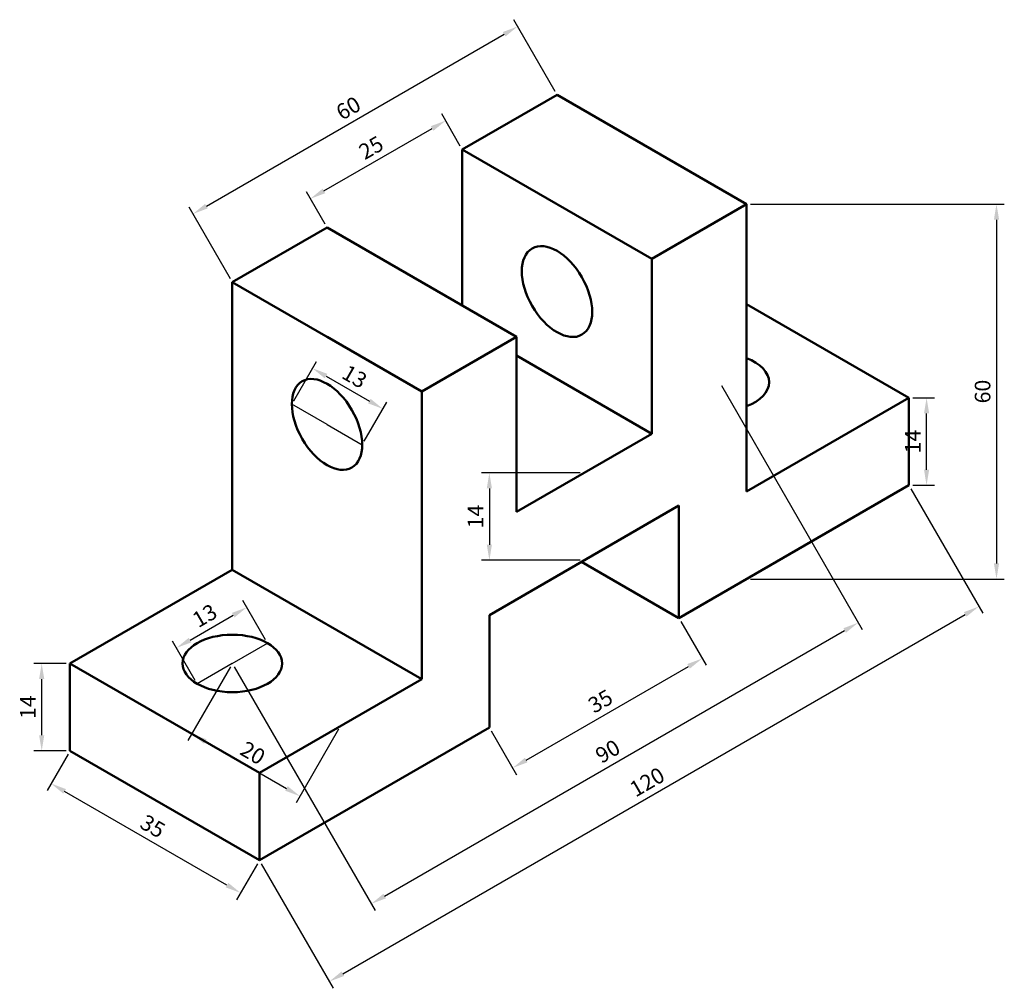
# Model space of a CAD drawing. Units: millimetres. Extents: x -27 to 130, y 19 to 174.
import ezdxf

# ---------------------------------------------------------------- set-up
doc = ezdxf.new("R2010")
doc.units = ezdxf.units.MM
doc.layers.add('M-DIMS', color=2, linetype='Continuous', lineweight=25)
doc.layers.add('M-OUTL', color=7, linetype='Continuous', lineweight=50)
doc.styles.get("Standard").update_dxf_attribs({"font": 'arial.ttf'})
doc.dimstyles.new('ISO-25', dxfattribs={"dimtxt": 2.5, "dimasz": 2.5, "dimexe": 1.25, "dimexo": 0.625, "dimtad": 1, "dimtxsty": 'Standard', "dimcen": 2.5, "dimadec": 0, "dimazin": 0, "dimtfac": 1, "dimtmove": 0, "dimatfit": 3, "dimfxl": 1, "dimarcsym": 0})

# ---------------------------------------------------------------- blocks, each defined once
blk = doc.blocks.new('*D1')
at = {"layer": 'Defpoints', "color": 0, "transparency": 16777216}
for p in [(78.26, 78.03), (81.99, 71.56), (47.95, 60.53)]:
    blk.add_point(p, dxfattribs=at)
at = {"layer": 'M-DIMS', "color": 0, "lineweight": -2, "transparency": 16777216}
for p, q in [((78.57, 77.49), (82.62, 70.48)), ((53.84, 55.31), (79.83, 70.31)), ((48.26, 59.99), (52.3, 52.98))]:
    blk.add_line(p, q, dxfattribs=at)
at = {"layer": 'M-DIMS', "color": 0, "transparency": 16777216}
for points in [[(79.62, 70.68), (80.03, 69.95), (81.99, 71.56)], [(53.64, 55.68), (54.05, 54.95), (51.68, 54.06)]]:
    blk.add_solid(points, dxfattribs=at)
at = {"layer": 'M-DIMS', "color": 0, "transparency": 16777216, "insert": (65.88, 64.46), "char_height": 2.5, "attachment_point": 5, "rotation": 30}
blk.add_mtext('35', dxfattribs=at)
blk = doc.blocks.new('*D2')
at = {"layer": 'Defpoints', "color": 0, "transparency": 16777216}
for p in [(115.06, 113.28), (117.91, 113.28), (115.06, 99.28)]:
    blk.add_point(p, dxfattribs=at)
at = {"layer": 'M-DIMS', "color": 0, "lineweight": -2, "transparency": 16777216}
for p, q in [((115.69, 113.28), (119.16, 113.28)), ((117.91, 101.78), (117.91, 110.78)), ((115.69, 99.28), (119.16, 99.28))]:
    blk.add_line(p, q, dxfattribs=at)
at = {"layer": 'M-DIMS', "color": 0, "transparency": 16777216}
for points in [[(117.5, 110.78), (118.33, 110.78), (117.91, 113.28)], [(117.5, 101.78), (118.33, 101.78), (117.91, 99.28)]]:
    blk.add_solid(points, dxfattribs=at)
at = {"layer": 'M-DIMS', "color": 0, "transparency": 16777216, "insert": (116.03, 106.28), "char_height": 2.5, "attachment_point": 5, "rotation": 90}
blk.add_mtext('14', dxfattribs=at)
blk = doc.blocks.new('*D3')
at = {"layer": 'Defpoints', "color": 0, "transparency": 16777216}
for p in [(84.75, 115.78), (106.97, 77.3), (6.81, 70.78)]:
    blk.add_point(p, dxfattribs=at)
at = {"layer": 'M-DIMS', "color": 0, "lineweight": -2, "transparency": 16777216}
for p, q in [((85.07, 115.24), (107.59, 76.22)), ((31.19, 33.55), (104.8, 76.05)), ((7.12, 70.24), (29.65, 31.22))]:
    blk.add_line(p, q, dxfattribs=at)
at = {"layer": 'M-DIMS', "color": 0, "transparency": 16777216}
for points in [[(104.6, 76.41), (105.01, 75.69), (106.97, 77.3)], [(30.98, 33.91), (31.4, 33.19), (29.03, 32.3)]]:
    blk.add_solid(points, dxfattribs=at)
at = {"layer": 'M-DIMS', "color": 0, "transparency": 16777216, "insert": (67.05, 56.44), "char_height": 2.5, "attachment_point": 5, "rotation": 30}
blk.add_mtext('90', dxfattribs=at)
blk = doc.blocks.new('*D4')
at = {"layer": 'Defpoints', "color": 0, "transparency": 16777216}
for p in [(115.06, 99.28), (126.26, 79.88), (11.14, 39.28)]:
    blk.add_point(p, dxfattribs=at)
at = {"layer": 'M-DIMS', "color": 0, "lineweight": -2, "transparency": 16777216}
for p, q in [((115.38, 98.74), (126.89, 78.8)), ((24.51, 21.13), (124.1, 78.63)), ((11.45, 38.74), (22.97, 18.8))]:
    blk.add_line(p, q, dxfattribs=at)
at = {"layer": 'M-DIMS', "color": 0, "transparency": 16777216}
for points in [[(123.89, 78.99), (124.31, 78.27), (126.26, 79.88)], [(24.3, 21.49), (24.71, 20.77), (22.34, 19.88)]]:
    blk.add_solid(points, dxfattribs=at)
at = {"layer": 'M-DIMS', "color": 0, "transparency": 16777216, "insert": (73.35, 51.53), "char_height": 2.5, "attachment_point": 5, "rotation": 30}
blk.add_mtext('120', dxfattribs=at)
blk = doc.blocks.new('*D5')
at = {"layer": 'Defpoints', "color": 0, "transparency": 16777216}
for p in [(16.34, 112.28), (30.9, 111.51), (27.6, 105.78)]:
    blk.add_point(p, dxfattribs=at)
at = {"layer": 'M-DIMS', "color": 0, "lineweight": -2, "transparency": 16777216}
for p, q in [((16.65, 112.82), (20.27, 119.09)), ((21.81, 116.76), (28.74, 112.76)), ((27.91, 106.32), (31.53, 112.59))]:
    blk.add_line(p, q, dxfattribs=at)
at = {"layer": 'M-DIMS', "color": 0, "transparency": 16777216}
for points in [[(22.02, 117.12), (21.6, 116.4), (19.64, 118.01)], [(28.95, 113.12), (28.53, 112.4), (30.9, 111.51)]]:
    blk.add_solid(points, dxfattribs=at)
at = {"layer": 'M-DIMS', "color": 0, "transparency": 16777216, "insert": (26.22, 116.4), "char_height": 2.5, "attachment_point": 5, "rotation": 330}
blk.add_mtext('13', dxfattribs=at)
blk = doc.blocks.new('*D6')
at = {"layer": 'Defpoints', "color": 0, "transparency": 16777216}
for p in [(63.1, 101.28), (47.95, 87.28), (63.1, 87.28)]:
    blk.add_point(p, dxfattribs=at)
at = {"layer": 'M-DIMS', "color": 0, "lineweight": -2, "transparency": 16777216}
for p, q in [((62.48, 101.28), (46.7, 101.28)), ((47.95, 98.78), (47.95, 89.78)), ((62.48, 87.28), (46.7, 87.28))]:
    blk.add_line(p, q, dxfattribs=at)
at = {"layer": 'M-DIMS', "color": 0, "transparency": 16777216}
for points in [[(47.53, 98.78), (48.36, 98.78), (47.95, 101.28)], [(47.53, 89.78), (48.36, 89.78), (47.95, 87.28)]]:
    blk.add_solid(points, dxfattribs=at)
at = {"layer": 'M-DIMS', "color": 0, "transparency": 16777216, "insert": (46.07, 94.28), "char_height": 2.5, "attachment_point": 5, "rotation": 90}
blk.add_mtext('14', dxfattribs=at)
blk = doc.blocks.new('*D7')
at = {"layer": 'Defpoints', "color": 0, "transparency": 16777216}
for p in [(9.13, 79.76), (12.44, 74.03), (1.18, 67.53)]:
    blk.add_point(p, dxfattribs=at)
at = {"layer": 'M-DIMS', "color": 0, "lineweight": -2, "transparency": 16777216}
for p, q in [((12.13, 74.57), (8.51, 80.84)), ((0.04, 74.51), (6.97, 78.51)), ((0.87, 68.07), (-2.75, 74.34))]:
    blk.add_line(p, q, dxfattribs=at)
at = {"layer": 'M-DIMS', "color": 0, "transparency": 16777216}
for points in [[(6.76, 78.87), (7.18, 78.15), (9.13, 79.76)], [(-0.17, 74.87), (0.25, 74.15), (-2.13, 73.26)]]:
    blk.add_solid(points, dxfattribs=at)
at = {"layer": 'M-DIMS', "color": 0, "transparency": 16777216, "insert": (2.55, 78.15), "char_height": 2.5, "attachment_point": 5, "rotation": 30}
blk.add_mtext('13', dxfattribs=at)
blk = doc.blocks.new('*D8')
at = {"layer": 'Defpoints', "color": 0, "transparency": 16777216}
for p in [(-23.69, 70.78), (-19.17, 70.78), (-19.17, 56.78)]:
    blk.add_point(p, dxfattribs=at)
at = {"layer": 'M-DIMS', "color": 0, "lineweight": -2, "transparency": 16777216}
for p, q in [((-19.8, 70.78), (-24.94, 70.78)), ((-23.69, 59.28), (-23.69, 68.28)), ((-19.8, 56.78), (-24.94, 56.78))]:
    blk.add_line(p, q, dxfattribs=at)
at = {"layer": 'M-DIMS', "color": 0, "transparency": 16777216}
for points in [[(-24.11, 68.28), (-23.28, 68.28), (-23.69, 70.78)], [(-24.11, 59.28), (-23.28, 59.28), (-23.69, 56.78)]]:
    blk.add_solid(points, dxfattribs=at)
at = {"layer": 'M-DIMS', "color": 0, "transparency": 16777216, "insert": (-25.57, 63.78), "char_height": 2.5, "attachment_point": 5, "rotation": 90}
blk.add_mtext('14', dxfattribs=at)
blk = doc.blocks.new('*D9')
at = {"layer": 'Defpoints', "color": 0, "transparency": 16777216}
for p in [(-19.17, 56.78), (-22.19, 51.56), (11.14, 39.28)]:
    blk.add_point(p, dxfattribs=at)
at = {"layer": 'M-DIMS', "color": 0, "lineweight": -2, "transparency": 16777216}
for p, q in [((-19.48, 56.24), (-22.81, 50.47)), ((5.96, 35.31), (-20.02, 50.31)), ((10.83, 38.74), (7.5, 32.97))]:
    blk.add_line(p, q, dxfattribs=at)
at = {"layer": 'M-DIMS', "color": 0, "transparency": 16777216}
for points in [[(-19.81, 50.67), (-20.23, 49.95), (-22.19, 51.56)], [(6.17, 35.67), (5.75, 34.95), (8.13, 34.06)]]:
    blk.add_solid(points, dxfattribs=at)
at = {"layer": 'M-DIMS', "color": 0, "transparency": 16777216, "insert": (-6.08, 44.45), "char_height": 2.5, "attachment_point": 5, "rotation": 330}
blk.add_mtext('35', dxfattribs=at)
blk = doc.blocks.new('*D10')
at = {"layer": 'Defpoints', "color": 0, "transparency": 16777216}
for p in [(6.81, 70.78), (24.13, 60.78), (17.64, 49.53)]:
    blk.add_point(p, dxfattribs=at)
at = {"layer": 'M-DIMS', "color": 0, "lineweight": -2, "transparency": 16777216}
for p, q in [((6.5, 70.24), (-0.31, 58.45)), ((23.82, 60.24), (17.01, 48.45)), ((2.48, 58.28), (15.47, 50.78))]:
    blk.add_line(p, q, dxfattribs=at)
at = {"layer": 'M-DIMS', "color": 0, "transparency": 16777216}
for points in [[(2.69, 58.64), (2.27, 57.92), (0.32, 59.53)], [(15.68, 51.14), (15.26, 50.42), (17.64, 49.53)]]:
    blk.add_solid(points, dxfattribs=at)
at = {"layer": 'M-DIMS', "color": 0, "transparency": 16777216, "insert": (9.93, 56.18), "char_height": 2.5, "attachment_point": 5, "rotation": 330}
blk.add_mtext('20', dxfattribs=at)
blk = doc.blocks.new('*D11')
at = {"layer": 'Defpoints', "color": 0, "transparency": 16777216}
for p in [(40.96, 157.63), (43.62, 153.03), (21.97, 140.53)]:
    blk.add_point(p, dxfattribs=at)
at = {"layer": 'M-DIMS', "color": 0, "lineweight": -2, "transparency": 16777216}
for p, q in [((43.3, 153.57), (40.33, 158.72)), ((21.47, 146.38), (38.79, 156.38)), ((21.65, 141.07), (18.68, 146.22))]:
    blk.add_line(p, q, dxfattribs=at)
at = {"layer": 'M-DIMS', "color": 0, "transparency": 16777216}
for points in [[(38.58, 156.75), (39, 156.02), (40.96, 157.63)], [(21.26, 146.75), (21.68, 146.02), (19.31, 145.13)]]:
    blk.add_solid(points, dxfattribs=at)
at = {"layer": 'M-DIMS', "color": 0, "transparency": 16777216, "insert": (29.18, 153.03), "char_height": 2.5, "attachment_point": 5, "rotation": 30}
blk.add_mtext('25', dxfattribs=at)
blk = doc.blocks.new('*D12')
at = {"layer": 'Defpoints', "color": 0, "transparency": 16777216}
for p in [(52.47, 172.7), (58.77, 161.78), (6.81, 131.78)]:
    blk.add_point(p, dxfattribs=at)
at = {"layer": 'M-DIMS', "color": 0, "lineweight": -2, "transparency": 16777216}
for p, q in [((58.46, 162.32), (51.84, 173.78)), ((2.67, 143.95), (50.3, 171.45)), ((6.5, 132.32), (-0.12, 143.78))]:
    blk.add_line(p, q, dxfattribs=at)
at = {"layer": 'M-DIMS', "color": 0, "transparency": 16777216}
for points in [[(50.09, 171.81), (50.51, 171.09), (52.47, 172.7)], [(2.46, 144.31), (2.88, 143.59), (0.51, 142.7)]]:
    blk.add_solid(points, dxfattribs=at)
at = {"layer": 'M-DIMS', "color": 0, "transparency": 16777216, "insert": (25.54, 159.35), "char_height": 2.5, "attachment_point": 5, "rotation": 30}
blk.add_mtext('60', dxfattribs=at)
blk = doc.blocks.new('*D13')
at = {"layer": 'Defpoints', "color": 0, "transparency": 16777216}
for p in [(89.08, 144.28), (89.08, 84.28), (129.1, 84.28)]:
    blk.add_point(p, dxfattribs=at)
at = {"layer": 'M-DIMS', "color": 0, "lineweight": -2, "transparency": 16777216}
for p, q in [((89.71, 144.28), (130.35, 144.28)), ((129.1, 141.78), (129.1, 86.78)), ((89.71, 84.28), (130.35, 84.28))]:
    blk.add_line(p, q, dxfattribs=at)
at = {"layer": 'M-DIMS', "color": 0, "transparency": 16777216}
for points in [[(128.69, 141.78), (129.52, 141.78), (129.1, 144.28)], [(128.69, 86.78), (129.52, 86.78), (129.1, 84.28)]]:
    blk.add_solid(points, dxfattribs=at)
at = {"layer": 'M-DIMS', "color": 0, "transparency": 16777216, "insert": (127.2, 114.28), "char_height": 2.5, "attachment_point": 5, "rotation": 90}
blk.add_mtext('60', dxfattribs=at)

msp = doc.modelspace()

# ---------------------------------------------------------------- linework, layer by layer
at = {"layer": 'M-DIMS'}
for p, q in [((21.966, 109.029), (16.337, 112.279)), ((21.966, 109.029), (27.595, 105.779)), ((6.811, 70.779), (12.44, 74.029)), ((6.811, 70.779), (1.181, 67.529))]:
    msp.add_line(p, q, dxfattribs=at)
at = {"layer": 'M-OUTL'}
for p, q in [((43.617, 153.029), (58.772, 161.779)), ((89.083, 144.279), (58.772, 161.779)), ((73.928, 135.529), (43.617, 153.029)), ((43.617, 153.029), (43.617, 128.029)), ((73.928, 135.529), (89.083, 144.279)), ((89.083, 144.279), (89.083, 98.279)), ((21.966, 140.529), (6.811, 131.779)), ((52.277, 123.029), (21.966, 140.529)), ((73.928, 107.529), (73.928, 135.529)), ((37.121, 114.279), (6.811, 131.779)), ((6.811, 131.779), (6.811, 85.779)), ((115.064, 113.279), (89.083, 128.279)), ((37.121, 114.279), (21.966, 123.029)), ((52.277, 123.029), (37.121, 114.279)), ((52.277, 95.029), (52.277, 123.029)), ((73.928, 107.529), (52.277, 120.029)), ((37.121, 114.279), (37.121, 68.279)), ((115.064, 113.279), (89.083, 98.279)), ((115.064, 99.279), (115.064, 113.279)), ((63.102, 101.279), (73.928, 107.529)), ((63.102, 101.279), (52.277, 95.029)), ((78.258, 78.029), (115.064, 99.279)), ((78.258, 96.029), (47.947, 78.529)), ((78.258, 78.029), (78.258, 96.029)), ((78.258, 78.029), (62.669, 87.029)), ((6.811, 85.779), (-19.17, 70.779)), ((37.121, 68.279), (6.811, 85.779)), ((47.947, 78.529), (47.947, 60.529)), ((-19.17, 56.779), (-19.17, 70.779)), ((-19.17, 70.779), (11.141, 53.279)), ((11.141, 53.279), (37.121, 68.279)), ((47.947, 60.529), (11.141, 39.279)), ((11.141, 39.279), (-19.17, 56.779)), ((11.141, 39.279), (11.141, 53.279))]:
    msp.add_line(p, q, dxfattribs=at)
for centre, major_axis in [((58.772, 130.279), (3.98, -6.894)), ((21.966, 109.029), (3.98, -6.894)), ((6.811, 70.779), (-7.961, 0))]:
    msp.add_ellipse(centre, major_axis=major_axis, ratio=0.5773503, dxfattribs=at)
msp.add_ellipse((84.753, 115.779), major_axis=(-7.961, 0), ratio=0.5773503, start_param=2.1459078, end_param=4.1372776, dxfattribs=at)

# ---------------------------------------------------------------- dimensions: what is measured, and where the dimension line sits
at = {"layer": 'M-DIMS'}
for p1, p2, distance, picture, middle in [((6.811, 131.779), (58.772, 161.779), 12.611, '*D12', (25.535, 159.347)), ((21.966, 140.529), (43.617, 153.029), 5.318, '*D11', (29.182, 153.031)), ((16.337, 112.279), (27.595, 105.779), 6.613, '*D5', (26.224, 116.404)), ((6.811, 70.779), (84.753, 115.779), -44.434, '*D3', (67.048, 56.445)), ((11.141, 39.279), (115.064, 99.279), -22.401, '*D4', (73.352, 51.526)), ((1.181, 67.529), (12.44, 74.029), 6.614, '*D7', (2.552, 78.155)), ((47.947, 60.529), (78.258, 78.029), -7.465, '*D1', (65.883, 64.462)), ((6.811, 70.779), (24.131, 60.779), -12.99, '*D10', (9.926, 56.176)), ((11.141, 39.279), (-19.17, 56.779), 6.031, '*D9', (-6.079, 44.454))]:
    dim = msp.add_aligned_dim(p1=p1, p2=p2, distance=distance, dimstyle='ISO-25', override={"dimclrd": 0, "dimclre": 0, "dimclrt": 0}, dxfattribs=at)
    dim.commit()
    dim.dimension.update_dxf_attribs({"geometry": picture, "text_midpoint": middle})
for base, p1, p2, picture, middle in [((129.103, 84.279), (89.083, 144.279), (89.083, 84.279), '*D13', (127.201, 114.279)), ((117.913, 113.279), (115.064, 99.279), (115.064, 113.279), '*D2', (116.033, 106.279)), ((47.947, 87.279), (63.102, 101.279), (63.102, 87.279), '*D6', (46.067, 94.279)), ((-23.694, 70.779), (-19.17, 56.779), (-19.17, 70.779), '*D8', (-25.574, 63.779))]:
    dim = msp.add_linear_dim(base=base, p1=p1, p2=p2, angle=90, dimstyle='ISO-25', override={"dimclrd": 0, "dimclre": 0, "dimclrt": 0}, dxfattribs=at)
    dim.commit()
    dim.dimension.update_dxf_attribs({"geometry": picture, "text_midpoint": middle})

doc.saveas('drawing.dxf')
